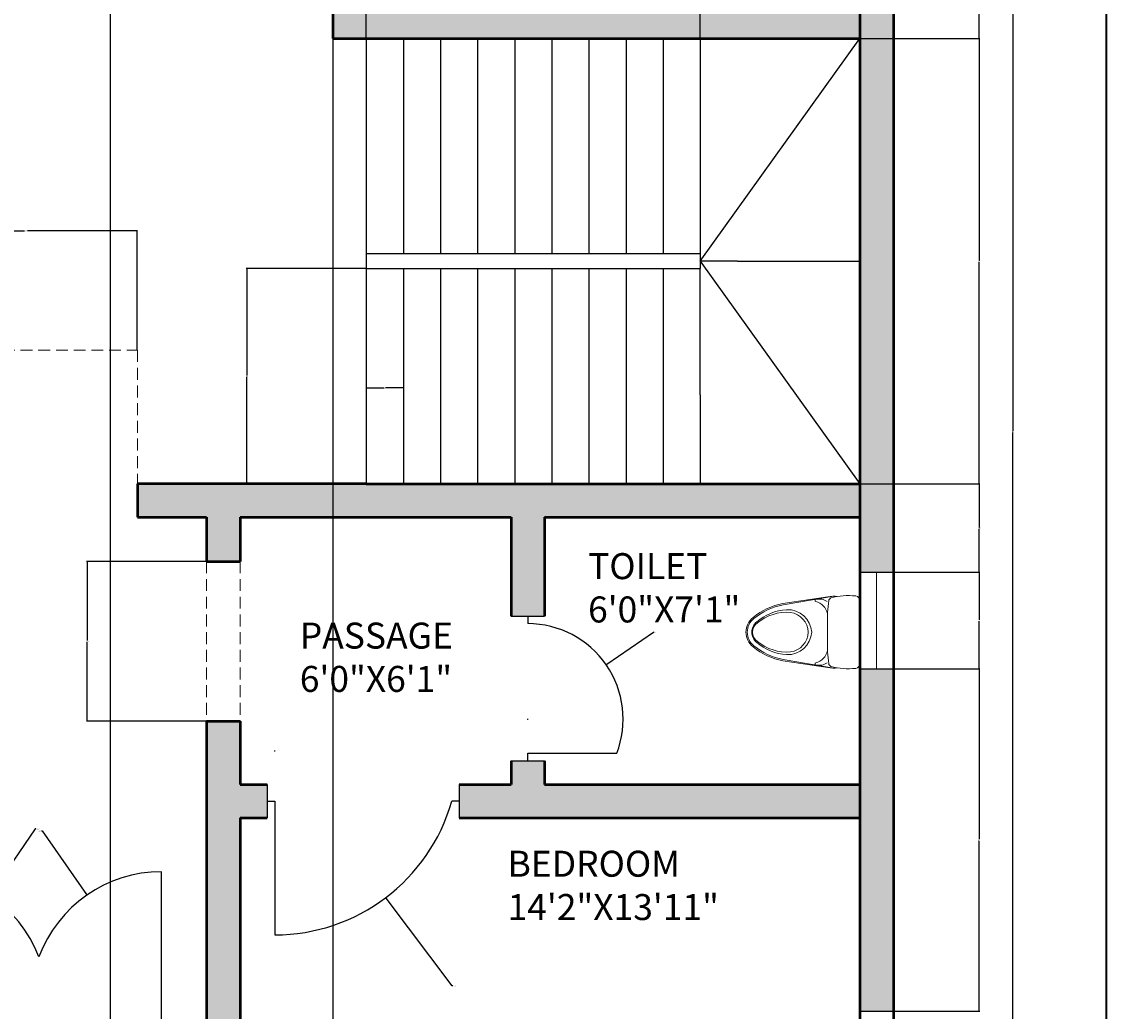
# Model space of a CAD drawing. Units: inches. Extents: x 1676 to 2199, y 1657 to 2783.
# Tile 7 of 10: x 1907 to 2199, y 1905 to 2172. Entities that reach past the tile are written whole.
import ezdxf

# ---------------------------------------------------------------- set-up
doc = ezdxf.new("R2010")
doc.units = ezdxf.units.IN
doc.linetypes.add('HIDDEN2', pattern=[4.7625, 3.175, -1.5875])
for name, color, linetype, lineweight in [('A-ANNO-DIMS', 2, 'Continuous', 18), ('A-ANNO-TTLB', 7, 'Continuous', 35), ('A-AREA-IDEN', 7, 'Continuous', 18), ('A-DOOR', 4, 'Continuous', 25), ('A-FLOR-FIXT', 9, 'Continuous', 18), ('A-FLOR-STRS', 7, 'Continuous', 25), ('A-GLAZ', 4, 'Continuous', 18), ('A-WALL', 7, 'Continuous', 50), ('A-WALL-HIDN', 253, 'HIDDEN2', 18)]:
    doc.layers.add(name, color=color, linetype=linetype, lineweight=lineweight)
doc.layers.add('A-WALL-PATT', color=251, linetype='Continuous', lineweight=13, true_color=0x636466)
doc.styles.get("Standard").update_dxf_attribs({"font": 'arial.ttf'})
doc.dimstyles.get("Standard").update_dxf_attribs({"dimtxt": 0.18, "dimasz": 0.18, "dimexe": 0.18, "dimexo": 0.0625, "dimgap": 0.09, "dimtad": 0, "dimtih": 1, "dimtoh": 1, "dimdec": 4, "dimzin": 0, "dimdsep": 46, "dimtxsty": 'Standard', "dimcen": 0.09, "dimadec": 0, "dimazin": 0, "dimtfac": 1, "dimtdec": 4, "dimtofl": 0, "dimtmove": 0, "dimatfit": 3, "dimfxl": 1, "dimtolj": 1, "dimtzin": 0, "dimarcsym": 0})

# ---------------------------------------------------------------- blocks, each defined once
blk = doc.blocks.new('A$C188A4A68')
at = {"ltscale": 20}
for p, q in [((0.2444, 0.7693), (0.0344, 0.7693)), ((0.2444, 0.7693), (0.4544, 0.7693)), ((0.0013, 0.5938), (0.0607, 0.2504)), ((0.4874, 0.5938), (0.428, 0.2504)), ((0.0054, 0.5515), (0.0519, 0.2489)), ((0.2444, 0.5498), (0.1889, 0.5498)), ((0.2444, 0.5498), (0.2998, 0.5498)), ((0.4833, 0.5515), (0.4368, 0.2489))]:
    blk.add_line(p, q, dxfattribs=at)
for centre, radius, start, end in [((0.442, 0.6914), 0.4447, 173.63949, 195.46404), ((0.0344, 0.7343), 0.0349, 90, 169.59261), ((0.4544, 0.7343), 0.0349, 10.40739, 90), ((0.0467, 0.6914), 0.4447, 344.53596, 6.36051), ((0.2125, 0.5932), 0.2113, 172.64979, 191.36585), ((0.2762, 0.5932), 0.2113, 348.63415, 7.35021), ((0.0333, 0.5802), 0.0213, 200.24298, 267.15028), ((0.1303, 0.4913), 0.1097, 148.50689, 190.04883), ((0.1632, 1.4554), 0.906, 261.69023, 271.62576), ((0.1461, 0.4405), 0.1134, 104.10408, 164.15012), ((0.3255, 1.4554), 0.906, 268.37424, 278.30977), ((0.3426, 0.4405), 0.1134, 15.84988, 75.89592), ((0.3584, 0.4913), 0.1097, 349.95117, 31.49311), ((0.4554, 0.5802), 0.0213, 272.84972, 339.75702), ((0.0297, 0.4734), 0.0075, 189.82636, 345.08753), ((0.254, 0.2824), 0.1613, 93.43328, 183.00378), ((0.2347, 0.2824), 0.1613, 356.99622, 86.56672), ((0.459, 0.4734), 0.0075, 194.91247, 350.17364), ((0.2493, 0.2813), 0.1393, 92.03292, 172.03731), ((0.2394, 0.2813), 0.1393, 7.96269, 87.96708), ((0.4211, 0.2752), 0.3108, 175.32131, 219.24773), ((0.0676, 0.2752), 0.3108, 320.75227, 4.67869), ((0.4781, 0.3243), 0.4328, 190.02971, 219.74275), ((0.4781, 0.3243), 0.4238, 190.04347, 219.7538), ((0.4311, 0.2946), 0.3389, 183.50421, 221.02292), ((0.0576, 0.2946), 0.3389, 318.97708, 356.49579), ((0.0106, 0.3243), 0.4238, 320.2462, 349.95653), ((0.0106, 0.3243), 0.4328, 320.25725, 349.97029), ((0.2498, 0.1282), 0.0854, 215.56846, 266.31968), ((0.2389, 0.1282), 0.0854, 273.68032, 324.43154), ((0.2444, 0.127), 0.127, 218.71605, 270), ((0.2444, 0.127), 0.118, 218.67741, 270), ((0.2444, 0.127), 0.088, 218.504, 270), ((0.2444, 0.127), 0.088, 270, 321.496), ((0.2444, 0.127), 0.118, 270, 321.32259), ((0.2444, 0.127), 0.127, 270, 321.28395)]:
    blk.add_arc(centre, radius, start, end, dxfattribs=at)
blk = doc.blocks.new('*D20')
at = {"layer": 'A-ANNO-DIMS', "color": 0, "lineweight": -2, "transparency": 16777216}
for p, q in [((2142.14, 2341.09), (2174.4, 2341.09)), ((2174.22, 2340.91), (2174.22, 2061.27)), ((2174.22, 1781.27), (2174.22, 2060.91)), ((2142.14, 1781.09), (2174.4, 1781.09))]:
    blk.add_line(p, q, dxfattribs=at)
at = {"layer": 'A-ANNO-DIMS', "color": 0, "transparency": 16777216}
for points in [[(2174.19, 2340.91), (2174.25, 2340.91), (2174.22, 2341.09)], [(2174.19, 1781.27), (2174.25, 1781.27), (2174.22, 1781.09)]]:
    blk.add_solid(points, dxfattribs=at)
at = {"layer": 'Defpoints', "color": 0, "transparency": 16777216}
for p in [(2142.07, 2341.09), (2174.22, 2341.09), (2142.07, 1781.09)]:
    blk.add_point(p, dxfattribs=at)
at = {"layer": 'A-ANNO-DIMS', "color": 0, "transparency": 16777216, "insert": (2174.22, 2061.09), "char_height": 0.18, "attachment_point": 5}
blk.add_mtext('\\A1;560', dxfattribs=at)
blk = doc.blocks.new('*D31')
at = {"layer": 'A-ANNO-DIMS', "color": 0, "lineweight": -2, "transparency": 16777216}
for p, q in [((2133.14, 1997.28), (2165.4, 1997.28)), ((2165.22, 1997.1), (2165.22, 1951.32)), ((2165.22, 1905.17), (2165.22, 1950.95)), ((2133.14, 1904.99), (2165.4, 1904.99))]:
    blk.add_line(p, q, dxfattribs=at)
at = {"layer": 'A-ANNO-DIMS', "color": 0, "transparency": 16777216}
for points in [[(2165.19, 1997.1), (2165.25, 1997.1), (2165.22, 1997.28)], [(2165.19, 1905.17), (2165.25, 1905.17), (2165.22, 1904.99)]]:
    blk.add_solid(points, dxfattribs=at)
at = {"layer": 'Defpoints', "color": 0, "transparency": 16777216}
for p in [(2133.07, 1997.28), (2133.07, 1904.99), (2165.22, 1904.99)]:
    blk.add_point(p, dxfattribs=at)
at = {"layer": 'A-ANNO-DIMS', "color": 0, "transparency": 16777216, "insert": (2165.22, 1951.13), "char_height": 0.18, "attachment_point": 5}
blk.add_mtext('\\A1;92.29', dxfattribs=at)
blk = doc.blocks.new('*D32')
at = {"layer": 'A-ANNO-DIMS', "color": 0, "lineweight": -2, "transparency": 16777216}
for p, q in [((2133.14, 2023.28), (2165.4, 2023.28)), ((2165.22, 2023.1), (2165.22, 2010.46)), ((2165.22, 1997.46), (2165.22, 2010.1)), ((2133.14, 1997.28), (2165.4, 1997.28))]:
    blk.add_line(p, q, dxfattribs=at)
at = {"layer": 'A-ANNO-DIMS', "color": 0, "transparency": 16777216}
for points in [[(2165.19, 2023.1), (2165.25, 2023.1), (2165.22, 2023.28)], [(2165.19, 1997.46), (2165.25, 1997.46), (2165.22, 1997.28)]]:
    blk.add_solid(points, dxfattribs=at)
at = {"layer": 'Defpoints', "color": 0, "transparency": 16777216}
for p in [(2133.07, 2023.28), (2133.07, 1997.28), (2165.22, 1997.28)]:
    blk.add_point(p, dxfattribs=at)
at = {"layer": 'A-ANNO-DIMS', "color": 0, "transparency": 16777216, "insert": (2165.22, 2010.28), "char_height": 0.18, "attachment_point": 5}
blk.add_mtext('\\A1;26', dxfattribs=at)
blk = doc.blocks.new('*D33')
at = {"layer": 'A-ANNO-DIMS', "color": 0, "lineweight": -2, "transparency": 16777216}
for p, q in [((2133.14, 2047.09), (2165.4, 2047.09)), ((2165.22, 2046.91), (2165.22, 2035.36)), ((2165.22, 2023.46), (2165.22, 2035)), ((2133.14, 2023.28), (2165.4, 2023.28))]:
    blk.add_line(p, q, dxfattribs=at)
at = {"layer": 'A-ANNO-DIMS', "color": 0, "transparency": 16777216}
for points in [[(2165.19, 2046.91), (2165.25, 2046.91), (2165.22, 2047.09)], [(2165.19, 2023.46), (2165.25, 2023.46), (2165.22, 2023.28)]]:
    blk.add_solid(points, dxfattribs=at)
at = {"layer": 'Defpoints', "color": 0, "transparency": 16777216}
for p in [(2133.07, 2047.09), (2133.07, 2023.28), (2165.22, 2023.28)]:
    blk.add_point(p, dxfattribs=at)
at = {"layer": 'A-ANNO-DIMS', "color": 0, "transparency": 16777216, "insert": (2165.22, 2035.18), "char_height": 0.18, "attachment_point": 5}
blk.add_mtext('\\A1;23.81', dxfattribs=at)
blk = doc.blocks.new('*D34')
at = {"layer": 'A-ANNO-DIMS', "color": 0, "lineweight": -2, "transparency": 16777216}
for p, q in [((2133.14, 2167.09), (2165.4, 2167.09)), ((2165.22, 2166.91), (2165.22, 2107.27)), ((2165.22, 2047.27), (2165.22, 2106.91)), ((2133.14, 2047.09), (2165.4, 2047.09))]:
    blk.add_line(p, q, dxfattribs=at)
at = {"layer": 'A-ANNO-DIMS', "color": 0, "transparency": 16777216}
for points in [[(2165.19, 2166.91), (2165.25, 2166.91), (2165.22, 2167.09)], [(2165.19, 2047.27), (2165.25, 2047.27), (2165.22, 2047.09)]]:
    blk.add_solid(points, dxfattribs=at)
at = {"layer": 'Defpoints', "color": 0, "transparency": 16777216}
for p in [(2133.07, 2167.09), (2133.07, 2047.09), (2165.22, 2047.09)]:
    blk.add_point(p, dxfattribs=at)
at = {"layer": 'A-ANNO-DIMS', "color": 0, "transparency": 16777216, "insert": (2165.22, 2107.09), "char_height": 0.18, "attachment_point": 5}
blk.add_mtext('\\A1;120', dxfattribs=at)
blk = doc.blocks.new('*D35')
at = {"layer": 'A-ANNO-DIMS', "color": 0, "lineweight": -2, "transparency": 16777216}
for p, q in [((2133.14, 2238.21), (2165.4, 2238.21)), ((2165.22, 2238.03), (2165.22, 2202.83)), ((2165.22, 2167.27), (2165.22, 2202.47)), ((2133.14, 2167.09), (2165.4, 2167.09))]:
    blk.add_line(p, q, dxfattribs=at)
at = {"layer": 'A-ANNO-DIMS', "color": 0, "transparency": 16777216}
for points in [[(2165.19, 2238.03), (2165.25, 2238.03), (2165.22, 2238.21)], [(2165.19, 2167.27), (2165.25, 2167.27), (2165.22, 2167.09)]]:
    blk.add_solid(points, dxfattribs=at)
at = {"layer": 'Defpoints', "color": 0, "transparency": 16777216}
for p in [(2133.07, 2238.21), (2133.07, 2167.09), (2165.22, 2167.09)]:
    blk.add_point(p, dxfattribs=at)
at = {"layer": 'A-ANNO-DIMS', "color": 0, "transparency": 16777216, "insert": (2165.22, 2202.65), "char_height": 0.18, "attachment_point": 5}
blk.add_mtext('\\A1;71.12', dxfattribs=at)
blk = doc.blocks.new('*D40')
at = {"layer": 'A-ANNO-DIMS', "color": 0, "lineweight": -2, "transparency": 16777216}
for p, q in [((1931.07, 2236.02), (1931.07, 1695.28)), ((1991.07, 2236.02), (1991.07, 1695.28)), ((1931.25, 1695.46), (1960.86, 1695.46)), ((1990.89, 1695.46), (1961.29, 1695.46))]:
    blk.add_line(p, q, dxfattribs=at)
at = {"layer": 'A-ANNO-DIMS', "color": 0, "transparency": 16777216}
for points in [[(1931.25, 1695.49), (1931.25, 1695.43), (1931.07, 1695.46)], [(1990.89, 1695.49), (1990.89, 1695.43), (1991.07, 1695.46)]]:
    blk.add_solid(points, dxfattribs=at)
at = {"layer": 'Defpoints', "color": 0, "transparency": 16777216}
for p in [(1931.07, 2236.09), (1991.07, 2236.09), (1991.07, 1695.46)]:
    blk.add_point(p, dxfattribs=at)
at = {"layer": 'A-ANNO-DIMS', "color": 0, "transparency": 16777216, "insert": (1961.07, 1695.46), "char_height": 0.18, "attachment_point": 5}
blk.add_mtext('\\A1;60', dxfattribs=at)
blk = doc.blocks.new('*D45')
at = {"layer": 'A-ANNO-DIMS', "color": 0, "lineweight": -2, "transparency": 16777216}
for p, q in [((2000.07, 2167.15), (2000.07, 2199.42)), ((2000.25, 2199.24), (2044.86, 2199.24)), ((2089.89, 2199.24), (2045.29, 2199.24)), ((2090.07, 2167.15), (2090.07, 2199.42))]:
    blk.add_line(p, q, dxfattribs=at)
at = {"layer": 'A-ANNO-DIMS', "color": 0, "transparency": 16777216}
for points in [[(2000.25, 2199.27), (2000.25, 2199.21), (2000.07, 2199.24)], [(2089.89, 2199.27), (2089.89, 2199.21), (2090.07, 2199.24)]]:
    blk.add_solid(points, dxfattribs=at)
at = {"layer": 'Defpoints', "color": 0, "transparency": 16777216}
for p in [(2090.07, 2199.24), (2000.07, 2167.09), (2090.07, 2167.09)]:
    blk.add_point(p, dxfattribs=at)
at = {"layer": 'A-ANNO-DIMS', "color": 0, "transparency": 16777216, "insert": (2045.07, 2199.24), "char_height": 0.18, "attachment_point": 5}
blk.add_mtext('\\A1;90', dxfattribs=at)
blk = doc.blocks.new('*D46')
at = {"layer": 'A-ANNO-DIMS', "color": 0, "lineweight": -2, "transparency": 16777216}
for p, q in [((2090.07, 2167.15), (2090.07, 2199.42)), ((2090.25, 2199.24), (2111.35, 2199.24)), ((2132.89, 2199.24), (2111.8, 2199.24)), ((2133.07, 2167.15), (2133.07, 2199.42))]:
    blk.add_line(p, q, dxfattribs=at)
at = {"layer": 'A-ANNO-DIMS', "color": 0, "transparency": 16777216}
for points in [[(2090.25, 2199.27), (2090.25, 2199.21), (2090.07, 2199.24)], [(2132.89, 2199.27), (2132.89, 2199.21), (2133.07, 2199.24)]]:
    blk.add_solid(points, dxfattribs=at)
at = {"layer": 'Defpoints', "color": 0, "transparency": 16777216}
for p in [(2133.07, 2199.24), (2090.07, 2167.09), (2133.07, 2167.09)]:
    blk.add_point(p, dxfattribs=at)
at = {"layer": 'A-ANNO-DIMS', "color": 0, "transparency": 16777216, "insert": (2111.57, 2199.24), "char_height": 0.18, "attachment_point": 5}
blk.add_mtext('\\A1;43', dxfattribs=at)
blk = doc.blocks.new('*D47')
at = {"layer": 'A-ANNO-DIMS', "color": 0, "lineweight": -2, "transparency": 16777216}
for p, q in [((2000.01, 2105.09), (1967.74, 2105.09)), ((1967.92, 2104.91), (1967.92, 2076.27)), ((1967.92, 2047.27), (1967.92, 2075.91)), ((2000.01, 2047.09), (1967.74, 2047.09))]:
    blk.add_line(p, q, dxfattribs=at)
at = {"layer": 'A-ANNO-DIMS', "color": 0, "transparency": 16777216}
for points in [[(1967.89, 2104.91), (1967.95, 2104.91), (1967.92, 2105.09)], [(1967.89, 2047.27), (1967.95, 2047.27), (1967.92, 2047.09)]]:
    blk.add_solid(points, dxfattribs=at)
at = {"layer": 'Defpoints', "color": 0, "transparency": 16777216}
for p in [(1967.92, 2105.09), (2000.07, 2105.09), (2000.07, 2047.09)]:
    blk.add_point(p, dxfattribs=at)
at = {"layer": 'A-ANNO-DIMS', "color": 0, "transparency": 16777216, "insert": (1967.92, 2076.09), "char_height": 0.18, "attachment_point": 5}
blk.add_mtext('\\A1;58', dxfattribs=at)
blk = doc.blocks.new('*D48')
at = {"layer": 'A-ANNO-DIMS', "color": 0, "lineweight": -2, "transparency": 16777216}
for p, q in [((2000.07, 2105.02), (2000.07, 2072.76)), ((2010.07, 2105.02), (2010.07, 2072.76)), ((2000.25, 2072.94), (2004.86, 2072.94)), ((2009.89, 2072.94), (2005.29, 2072.94))]:
    blk.add_line(p, q, dxfattribs=at)
at = {"layer": 'A-ANNO-DIMS', "color": 0, "transparency": 16777216}
for points in [[(2000.25, 2072.97), (2000.25, 2072.91), (2000.07, 2072.94)], [(2009.89, 2072.97), (2009.89, 2072.91), (2010.07, 2072.94)]]:
    blk.add_solid(points, dxfattribs=at)
at = {"layer": 'Defpoints', "color": 0, "transparency": 16777216}
for p in [(2000.07, 2105.09), (2010.07, 2105.09), (2000.07, 2072.94)]:
    blk.add_point(p, dxfattribs=at)
at = {"layer": 'A-ANNO-DIMS', "color": 0, "transparency": 16777216, "insert": (2005.07, 2072.94), "char_height": 0.18, "attachment_point": 5}
blk.add_mtext('\\A1;10', dxfattribs=at)
blk = doc.blocks.new('*D49')
at = {"layer": 'A-ANNO-DIMS', "color": 0, "lineweight": -2, "transparency": 16777216}
for p, q in [((1878.39, 2083.15), (1878.39, 2115.42)), ((1878.57, 2115.24), (1908.02, 2115.24)), ((1938.22, 2115.24), (1908.78, 2115.24)), ((1938.4, 2083.15), (1938.4, 2115.42))]:
    blk.add_line(p, q, dxfattribs=at)
at = {"layer": 'A-ANNO-DIMS', "color": 0, "transparency": 16777216}
for points in [[(1878.57, 2115.27), (1878.57, 2115.21), (1878.39, 2115.24)], [(1938.22, 2115.27), (1938.22, 2115.21), (1938.4, 2115.24)]]:
    blk.add_solid(points, dxfattribs=at)
at = {"layer": 'Defpoints', "color": 0, "transparency": 16777216}
for p in [(1938.4, 2115.24), (1878.39, 2083.09), (1938.4, 2083.09)]:
    blk.add_point(p, dxfattribs=at)
at = {"layer": 'A-ANNO-DIMS', "color": 0, "transparency": 16777216, "insert": (1908.4, 2115.24), "char_height": 0.18, "attachment_point": 5}
blk.add_mtext('\\A1;60.01', dxfattribs=at)
blk = doc.blocks.new('*D58')
at = {"layer": 'A-ANNO-DIMS', "color": 0, "lineweight": -2, "transparency": 16777216}
for p, q in [((1957.01, 2026.16), (1924.74, 2026.16)), ((1924.92, 2025.98), (1924.92, 2004.84)), ((1924.92, 1983.33), (1924.92, 2004.47)), ((1957.01, 1983.15), (1924.74, 1983.15))]:
    blk.add_line(p, q, dxfattribs=at)
at = {"layer": 'A-ANNO-DIMS', "color": 0, "transparency": 16777216}
for points in [[(1924.89, 2025.98), (1924.95, 2025.98), (1924.92, 2026.16)], [(1924.89, 1983.33), (1924.95, 1983.33), (1924.92, 1983.15)]]:
    blk.add_solid(points, dxfattribs=at)
at = {"layer": 'Defpoints', "color": 0, "transparency": 16777216}
for p in [(1924.92, 2026.16), (1957.07, 2026.16), (1957.07, 1983.15)]:
    blk.add_point(p, dxfattribs=at)
at = {"layer": 'A-ANNO-DIMS', "color": 0, "transparency": 16777216, "insert": (1924.92, 2004.66), "char_height": 0.18, "attachment_point": 5}
blk.add_mtext('\\A1;43.01', dxfattribs=at)
blk = doc.blocks.new('*D79')
at = {"layer": 'A-ANNO-DIMS', "color": 0, "lineweight": -2, "transparency": 16777216}
for p, q in [((2077.47, 2007.01), (2064.91, 1998.38)), ((2077.65, 2007.01), (2077.47, 2007.01)), ((2043.48, 1983.71), (2043.66, 1983.71)), ((2043.57, 1983.62), (2043.57, 1983.8))]:
    blk.add_line(p, q, dxfattribs=at)
at = {"layer": 'A-ANNO-DIMS', "color": 0, "transparency": 16777216}
blk.add_solid([(2064.89, 1998.4), (2064.93, 1998.35), (2064.76, 1998.28)], dxfattribs=at)
at = {"layer": 'Defpoints', "color": 0, "transparency": 16777216}
for p in [(2064.76, 1998.28), (2043.57, 1983.71)]:
    blk.add_point(p, dxfattribs=at)
at = {"layer": 'A-ANNO-DIMS', "color": 0, "transparency": 16777216, "insert": (2078.2, 2007.01), "char_height": 0.18, "attachment_point": 5}
blk.add_mtext('\\A1;R25.707', dxfattribs=at)
blk = doc.blocks.new('*D80')
at = {"layer": 'A-ANNO-DIMS', "color": 0, "lineweight": -2, "transparency": 16777216}
for p, q in [((1975.33, 1975.17), (1975.51, 1975.17)), ((1975.42, 1975.08), (1975.42, 1975.26)), ((2023.22, 1911.85), (2005.4, 1935.45)), ((2023.4, 1911.85), (2023.22, 1911.85))]:
    blk.add_line(p, q, dxfattribs=at)
at = {"layer": 'A-ANNO-DIMS', "color": 0, "transparency": 16777216}
blk.add_solid([(2005.43, 1935.47), (2005.38, 1935.44), (2005.29, 1935.6)], dxfattribs=at)
at = {"layer": 'Defpoints', "color": 0, "transparency": 16777216}
for p in [(1975.42, 1975.17), (2005.29, 1935.6)]:
    blk.add_point(p, dxfattribs=at)
at = {"layer": 'A-ANNO-DIMS', "color": 0, "transparency": 16777216, "insert": (2023.88, 1911.85), "char_height": 0.18, "attachment_point": 5}
blk.add_mtext('\\A1;R49.59', dxfattribs=at)
blk = doc.blocks.new('*D81')
at = {"layer": 'A-ANNO-DIMS', "color": 0, "lineweight": -2, "transparency": 16777216}
for p, q in [((1910.86, 1954.14), (1898.76, 1936.45)), ((1911.04, 1954.14), (1910.86, 1954.14)), ((1878.23, 1906.55), (1878.41, 1906.55)), ((1878.32, 1906.46), (1878.32, 1906.64))]:
    blk.add_line(p, q, dxfattribs=at)
at = {"layer": 'A-ANNO-DIMS', "color": 0, "transparency": 16777216}
blk.add_solid([(1898.73, 1936.46), (1898.78, 1936.43), (1898.66, 1936.3)], dxfattribs=at)
at = {"layer": 'Defpoints', "color": 0, "transparency": 16777216}
for p in [(1898.66, 1936.3), (1878.32, 1906.55)]:
    blk.add_point(p, dxfattribs=at)
at = {"layer": 'A-ANNO-DIMS', "color": 0, "transparency": 16777216, "insert": (1911.59, 1954.14), "char_height": 0.18, "attachment_point": 5}
blk.add_mtext('\\A1;R36.034', dxfattribs=at)
blk = doc.blocks.new('*D82')
at = {"layer": 'A-ANNO-DIMS', "color": 0, "lineweight": -2, "transparency": 16777216}
for p, q in [((1912.55, 1953.6), (1912.73, 1953.6)), ((1912.73, 1953.6), (1924.68, 1936.43)), ((1944.79, 1907.42), (1944.97, 1907.42)), ((1944.88, 1907.33), (1944.88, 1907.51))]:
    blk.add_line(p, q, dxfattribs=at)
at = {"layer": 'A-ANNO-DIMS', "color": 0, "transparency": 16777216}
blk.add_solid([(1924.71, 1936.45), (1924.66, 1936.41), (1924.78, 1936.28)], dxfattribs=at)
at = {"layer": 'Defpoints', "color": 0, "transparency": 16777216}
for p in [(1924.78, 1936.28), (1944.88, 1907.42)]:
    blk.add_point(p, dxfattribs=at)
at = {"layer": 'A-ANNO-DIMS', "color": 0, "transparency": 16777216, "insert": (1912.07, 1953.6), "char_height": 0.18, "attachment_point": 5}
blk.add_mtext('\\A1;R35.17', dxfattribs=at)

msp = doc.modelspace()

# ---------------------------------------------------------------- hatches: boundary and pattern name
at = {"layer": 'A-WALL-PATT'}
h = msp.add_hatch(color=256, dxfattribs=at)
h.dxf.hatch_style = 1
h.paths.add_polyline_path([(1945.4216, 2336.5871), (1945.4216, 2341.0871), (1755.075, 2341.0871), (1755.075, 2323.0739), (1764.075, 2323.0739), (1764.075, 2332.0871), (1945.4216, 2332.0871)])
h.paths.add_polyline_path([(1764.075, 2299.0739), (1755.075, 2299.0739), (1755.075, 2266.2601), (1759.575, 2266.2601), (1764.075, 2266.2601)])
h.paths.add_polyline_path([(1843.075, 2285.0871), (1764.075, 2285.0871), (1764.075, 2276.0871), (1843.075, 2276.0871)])
h.paths.add_polyline_path([(1931.075, 2332.0871), (1922.075, 2332.0871), (1922.075, 2285.0871), (1907.247, 2285.0871), (1907.247, 2276.0871), (1922.075, 2276.0871), (1922.075, 2263.0871), (1922.075, 2214.434), (1922.075, 2183.2198), (1931.075, 2183.2198), (1931.075, 2214.434), (1931.075, 2227.0871), (1991.075, 2227.0871), (1991.075, 2176.0871), (1991.075, 2167.0871), (2000.075, 2167.0871), (2133.075, 2167.0871), (2133.075, 2176.0871), (2000.075, 2176.0871), (2000.075, 2245.3418), (1995.575, 2245.3418), (1991.075, 2245.3418), (1991.075, 2236.0871), (1931.075, 2236.0871)])
h.paths.add_polyline_path([(2000.075, 2332.0871), (1991.075, 2332.0871), (1991.075, 2285.0871), (1991.075, 2274.6339), (2000.075, 2274.6339), (2000.075, 2285.0871)], flags=17)
h.paths.add_polyline_path([(2142.075, 2341.0871), (1969.4216, 2341.0871), (1969.4216, 2332.0871), (2133.075, 2332.0871), (2133.075, 2298.2101), (2142.075, 2298.2101)])
h.paths.add_polyline_path([(2142.075, 1844.9908), (2133.075, 1844.9908), (2133.075, 1790.0871), (2061.2106, 1790.0871), (2061.2106, 1781.0871), (2142.075, 1781.0871)])
h.paths.add_polyline_path([(2001.2106, 1790.0871), (1966.075, 1790.0871), (1966.075, 1957.0871), (1973.4183, 1957.0871), (1973.4183, 1966.0871), (1966.075, 1966.0871), (1966.075, 1983.1515), (1957.075, 1983.1515), (1957.075, 1899.0871), (1946.8789, 1899.0871), (1946.8789, 1890.0871), (1957.075, 1890.0871), (1957.075, 1781.0871), (2001.2106, 1781.0871), (2001.2106, 1785.5871)])
h.paths.add_polyline_path([(1876.3163, 1894.5871), (1876.3163, 1899.0871), (1820.9237, 1899.0871), (1820.9237, 1890.0871), (1876.3163, 1890.0871)])
h.paths.add_polyline_path([(1764.075, 2093.9207), (1759.575, 2093.9207), (1755.075, 2093.9207), (1755.075, 2019.5723), (1764.075, 2019.5723)])
h.paths.add_polyline_path([(1878.3926, 2083.0871), (1764.075, 2083.0871), (1764.075, 2074.0871), (1878.3926, 2074.0871)])
h.paths.add_polyline_path([(1764.075, 1959.5723), (1755.075, 1959.5723), (1755.075, 1890.0871), (1784.9237, 1890.0871), (1784.9237, 1894.5871), (1784.9237, 1899.0871), (1764.075, 1899.0871)])
h.paths.add_polyline_path([(2133.075, 2047.0871), (2000.075, 2047.0871), (1966.075, 2047.0871), (1957.075, 2047.0871), (1938.4046, 2047.0871), (1938.4046, 2038.0871), (1957.075, 2038.0871), (1957.075, 2026.1604), (1966.075, 2026.1604), (1966.075, 2038.0871), (2039.075, 2038.0871), (2039.075, 2011.4216), (2048.075, 2011.4216), (2048.075, 2038.0871), (2133.075, 2038.0871)])
h.paths.add_polyline_path([(2133.075, 1966.0871), (2048.075, 1966.0871), (2048.075, 1972.5045), (2039.075, 1972.5045), (2039.075, 1966.0871), (2025.1075, 1966.0871), (2025.1075, 1957.0871), (2133.075, 1957.0871)])
h.paths.add_polyline_path([(1764.075, 2206.2601), (1755.075, 2206.2601), (1755.075, 2153.9207), (1764.075, 2153.9207)])
h = msp.add_hatch(color=256, dxfattribs=at)
h.dxf.hatch_style = 1
h.paths.add_polyline_path([(2142.075, 2238.2101), (2133.075, 2238.2101), (2133.075, 2023.2789), (2142.075, 2023.2789)])
h.paths.add_polyline_path([(2142.075, 1997.2789), (2133.075, 1997.2789), (2133.075, 1904.9908), (2142.075, 1904.9908)])

# ---------------------------------------------------------------- linework, layer by layer
at = {"layer": 'A-ANNO-TTLB'}
msp.add_lwpolyline([(1676.2722, 2782.5054), (2199.4461, 2782.5054), (2199.4461, 1657.2705), (1676.2722, 1657.2705)], close=True, dxfattribs=at)
at = {"layer": 'A-DOOR'}
for p, q in [((2039.075, 2011.4216), (2048.075, 2011.4216)), ((2043.575, 2011.4216), (2043.575, 2009.4216)), ((2039.075, 1972.5045), (2048.075, 1972.5045)), ((2043.575, 1972.5045), (2043.575, 1974.5045)), ((2043.575, 1974.5045), (2067.575, 1974.5045)), ((1973.4183, 1966.0871), (1973.4183, 1957.0871)), ((2025.1075, 1966.0871), (2025.1075, 1957.0871)), ((1973.4183, 1961.5871), (1975.4183, 1961.5871)), ((1975.4183, 1961.5871), (1975.4183, 1925.5871)), ((2025.1075, 1961.5871), (2023.1075, 1961.5871)), ((1944.8789, 1894.5871), (1944.8789, 1942.5871))]:
    msp.add_line(p, q, dxfattribs=at)
for centre, radius, start, end in [((2043.575, 1983.7149), 25.7066, 339.004859, 90), ((1975.4183, 1975.174), 49.5869, 270, 344.097464), ((1878.3163, 1906.5528), 36.0343, 21.266188, 90), ((1944.8789, 1907.4201), 35.1669, 90, 159.697131)]:
    msp.add_arc(centre, radius, start, end, dxfattribs=at)
at = {"layer": 'A-FLOR-STRS'}
for p, q in [((2000.075, 2167.0871), (2000.075, 2071.0871)), ((2000.075, 2167.0871), (2000.075, 2107.0871)), ((2010.075, 2167.0871), (2010.075, 2109.0871)), ((2010.075, 2167.0871), (2010.075, 2109.0871)), ((2020.075, 2167.0871), (2020.075, 2109.0871)), ((2030.075, 2167.0871), (2030.075, 2109.0871)), ((2040.075, 2167.0871), (2040.075, 2109.0871)), ((2050.075, 2167.0871), (2050.075, 2109.0871)), ((2060.075, 2167.0871), (2060.075, 2109.0871)), ((2070.075, 2167.0871), (2070.075, 2109.0871)), ((2080.075, 2167.0871), (2080.075, 2109.0871)), ((2090.075, 2167.0871), (2090.075, 2109.0871)), ((2090.075, 2107.0871), (2133.075, 2167.0871)), ((2090.075, 2109.0871), (2000.075, 2109.0871)), ((2000.075, 2107.0871), (2000.075, 2105.0871)), ((2090.075, 2109.0871), (2090.075, 2105.0871)), ((2100.075, 2107.0871), (2090.075, 2107.0871)), ((2090.075, 2107.0871), (2133.075, 2047.0871)), ((2100.075, 2107.0871), (2133.075, 2107.0871)), ((2000.075, 2105.0871), (2090.075, 2105.0871)), ((2010.075, 2105.0871), (2010.075, 2071.0871)), ((2020.075, 2105.0871), (2020.075, 2047.0871)), ((2030.075, 2105.0871), (2030.075, 2047.0871)), ((2040.075, 2105.0871), (2040.075, 2047.0871)), ((2050.075, 2105.0871), (2050.075, 2047.0871)), ((2060.075, 2105.0871), (2060.075, 2047.0871)), ((2070.075, 2105.0871), (2070.075, 2047.0871)), ((2080.075, 2105.0871), (2080.075, 2047.0871)), ((2090.075, 2071.0871), (2090.075, 2105.0871)), ((2000.075, 2071.0871), (2000.075, 2047.0871)), ((2010.075, 2071.0871), (2010.075, 2047.0871)), ((2090.075, 2071.0871), (2090.075, 2047.0871))]:
    msp.add_line(p, q, dxfattribs=at)
at = {"layer": 'A-GLAZ'}
for p, q in [((2133.075, 2023.2789), (2142.075, 2023.2789)), ((2142.075, 2023.2789), (2137.575, 2023.2789)), ((2137.575, 2023.2789), (2137.575, 2021.2789)), ((2137.575, 2021.2789), (2137.575, 1997.2789)), ((2137.575, 1997.2789), (2133.075, 1997.2789)), ((2133.075, 1997.2789), (2142.075, 1997.2789))]:
    msp.add_line(p, q, dxfattribs=at)
at = {"layer": 'A-WALL'}
for p, q in [((2142.075, 2341.0871), (2142.075, 1781.0871)), ((2133.075, 2332.0871), (2133.075, 1790.0871)), ((1991.075, 2176.0871), (1991.075, 2167.0871)), ((1991.075, 2167.0871), (2000.075, 2167.0871)), ((2000.075, 2167.0871), (2133.075, 2167.0871)), ((1957.075, 2047.0871), (1938.4046, 2047.0871)), ((1938.4046, 2047.0871), (1938.4046, 2038.0871)), ((1966.075, 2047.0871), (1957.075, 2047.0871)), ((2000.075, 2047.0871), (1966.075, 2047.0871)), ((2000.075, 2047.0871), (2133.075, 2047.0871)), ((1938.4046, 2038.0871), (1957.075, 2038.0871)), ((1957.075, 2038.0871), (1957.075, 2026.1604)), ((1966.075, 2038.0871), (2039.075, 2038.0871)), ((1966.075, 2038.0871), (1966.075, 2026.1604)), ((1966.075, 2038.0871), (1966.075, 2026.1604)), ((1966.075, 2038.0871), (1966.075, 2038.0871)), ((1966.075, 2038.0871), (1966.075, 2026.1604)), ((2039.075, 2038.0871), (2039.075, 2011.4216)), ((2048.075, 2038.0871), (2048.075, 2011.4216)), ((2048.075, 2038.0871), (2133.075, 2038.0871)), ((1957.075, 2026.1604), (1966.075, 2026.1604)), ((1957.075, 1983.1515), (1966.075, 1983.1515)), ((1957.075, 1983.1515), (1957.075, 1899.0871)), ((1966.075, 1983.1515), (1966.075, 1966.0871)), ((1966.075, 1983.1515), (1966.075, 1966.0871)), ((1966.075, 1983.1515), (1966.075, 1966.0871)), ((2039.075, 1972.5045), (2039.075, 1966.0871)), ((2048.075, 1972.5045), (2048.075, 1966.0871)), ((1966.075, 1966.0871), (1973.4183, 1966.0871)), ((2025.1075, 1966.0871), (2039.075, 1966.0871)), ((2048.075, 1966.0871), (2133.075, 1966.0871)), ((1966.075, 1957.0871), (1973.4183, 1957.0871)), ((1966.075, 1957.0871), (1966.075, 1790.0871)), ((2025.1075, 1957.0871), (2133.075, 1957.0871))]:
    msp.add_line(p, q, dxfattribs=at)
at = {"layer": 'A-WALL-HIDN'}
for p, q in [((1878.3926, 2083.0871), (1938.4046, 2083.0871)), ((1938.4046, 2083.0871), (1938.4046, 2047.0871)), ((1957.075, 2026.1604), (1957.075, 1983.1515)), ((1966.075, 2026.1604), (1966.075, 1983.1515))]:
    msp.add_line(p, q, dxfattribs=at)

# ---------------------------------------------------------------- block references
at = {"layer": 'A-FLOR-FIXT', "xscale": 39.90803308922938, "yscale": 39.90803308922938, "zscale": 39.90803308922938, "rotation": 270}
msp.add_blockref('A$C188A4A68', (2102.3756, 2016.8789), dxfattribs=at)

# ---------------------------------------------------------------- texts
at = {"layer": 'A-AREA-IDEN', "char_height": 7, "attachment_point": 1}
for s, width, insert in [('TOILET\\P6\'0"X7\'1"', 69.101204, (2059.8306, 2028.4137)), ('PASSAGE\\P6\'0"X6\'1"', 70.288016, (1982.17, 2009.705)), ('BEDROOM\\P14\'2"X13\'11"', 94.929086, (2038.1459, 1948.2473))]:
    msp.add_mtext_dynamic_manual_height_columns(s, width=width, gutter_width=12.5, heights=[0], dxfattribs=dict(at, insert=insert))

# ---------------------------------------------------------------- dimensions: what is measured, and where the dimension line sits
at = {"layer": 'A-ANNO-DIMS'}
for base, p1, p2, angle, override, picture, middle in [((2174.225, 2341.0871), (2142.075, 1781.0871), (2142.075, 2341.0871), 90, {"dimdec": 0, "dimlfac": 1, "dimrnd": 0, "dimzin": 0, "dimdsep": 46, "dimlunit": 2}, '*D20', (2174.225, 2061.0871)), ((2165.225, 2167.0871), (2133.075, 2238.2101), (2133.075, 2167.0871), 270, {"dimdec": 2, "dimlfac": 1, "dimrnd": 0, "dimzin": 0, "dimdsep": 46, "dimlunit": 2}, '*D35', (2165.225, 2202.6486)), ((2090.075, 2199.2371), (2000.075, 2167.0871), (2090.075, 2167.0871), 0, {"dimdec": 0, "dimlfac": 1, "dimrnd": 0, "dimzin": 0, "dimdsep": 46, "dimlunit": 2}, '*D45', (2045.075, 2199.2371)), ((2165.225, 2047.0871), (2133.075, 2167.0871), (2133.075, 2047.0871), 270, {"dimdec": 0, "dimlfac": 1, "dimrnd": 0, "dimzin": 0, "dimdsep": 46, "dimlunit": 2}, '*D34', (2165.225, 2107.0871)), ((1967.925, 2105.0871), (2000.075, 2047.0871), (2000.075, 2105.0871), 90, {"dimdec": 0, "dimlfac": 1, "dimrnd": 0, "dimzin": 0, "dimdsep": 46, "dimlunit": 2}, '*D47', (1967.925, 2076.0871)), ((2000.075, 2072.9371), (2010.075, 2105.0871), (2000.075, 2105.0871), 180, {"dimdec": 0, "dimlfac": 1, "dimrnd": 0, "dimzin": 0, "dimdsep": 46, "dimlunit": 2}, '*D48', (2005.075, 2072.9371)), ((2165.225, 2023.2789), (2133.075, 2047.0871), (2133.075, 2023.2789), 270, {"dimdec": 2, "dimlfac": 1, "dimrnd": 0, "dimzin": 0, "dimdsep": 46, "dimlunit": 2}, '*D33', (2165.225, 2035.183)), ((1924.925, 2026.1604), (1957.075, 1983.1515), (1957.075, 2026.1604), 90, {"dimdec": 2, "dimlfac": 1, "dimrnd": 0, "dimzin": 0, "dimdsep": 46, "dimlunit": 2}, '*D58', (1924.925, 2004.6559)), ((2165.225, 1997.2789), (2133.075, 2023.2789), (2133.075, 1997.2789), 270, {"dimdec": 0, "dimlfac": 1, "dimrnd": 0, "dimzin": 0, "dimdsep": 46, "dimlunit": 2}, '*D32', (2165.225, 2010.2789)), ((2165.225, 1904.9908), (2133.075, 1997.2789), (2133.075, 1904.9908), 270, {"dimdec": 2, "dimlfac": 1, "dimrnd": 0, "dimzin": 0, "dimdsep": 46, "dimlunit": 2}, '*D31', (2165.225, 1951.1348))]:
    dim = msp.add_linear_dim(base=base, p1=p1, p2=p2, angle=angle, dimstyle='Standard', override=override, dxfattribs=at)
    dim.commit()
    dim.dimension.update_dxf_attribs({"geometry": picture, "text_midpoint": middle})
for base, p1, p2, override, picture, middle in [((1991.075, 1695.4613), (1931.075, 2236.0871), (1991.075, 2236.0871), {"dimdec": 0, "dimlfac": 1, "dimrnd": 0, "dimzin": 0, "dimdsep": 46, "dimlunit": 2}, '*D40', (1961.075, 1695.4613)), ((2133.075, 2199.2371), (2090.075, 2167.0871), (2133.075, 2167.0871), {"dimdec": 0, "dimlfac": 1, "dimrnd": 0, "dimzin": 0, "dimdsep": 46, "dimlunit": 2}, '*D46', (2111.575, 2199.2371)), ((1938.4046, 2115.2371), (1878.3926, 2083.0871), (1938.4046, 2083.0871), {"dimdec": 2, "dimlfac": 1, "dimrnd": 0, "dimzin": 0, "dimdsep": 46, "dimlunit": 2}, '*D49', (1908.3986, 2115.2371))]:
    dim = msp.add_linear_dim(base=base, p1=p1, p2=p2, dimstyle='Standard', override=override, dxfattribs=at)
    dim.commit()
    dim.dimension.update_dxf_attribs({"geometry": picture, "text_midpoint": middle})
for center, mpoint, override, picture, middle in [((2043.575, 1983.7149), (2064.76, 1998.276), {"dimdec": 3, "dimlfac": 1, "dimrnd": 0, "dimzin": 0, "dimdsep": 46, "dimlunit": 2}, '*D79', (2078.2008, 2007.0127)), ((1975.4183, 1975.174), (2005.2938, 1935.5973), {"dimdec": 2, "dimlfac": 1, "dimrnd": 0, "dimzin": 0, "dimdsep": 46, "dimlunit": 2}, '*D80', (2023.8791, 1911.8512)), ((1878.3163, 1906.5528), (1898.6571, 1936.2971), {"dimdec": 3, "dimlfac": 1, "dimrnd": 0, "dimzin": 0, "dimdsep": 46, "dimlunit": 2}, '*D81', (1911.5909, 1954.1437)), ((1944.8789, 1907.4201), (1924.7839, 1936.2802), {"dimdec": 2, "dimlfac": 1, "dimrnd": 0, "dimzin": 0, "dimdsep": 46, "dimlunit": 2}, '*D82', (1912.067, 1953.5962))]:
    dim = msp.add_radius_dim(center=center, mpoint=mpoint, dimstyle='Standard', override=override, dxfattribs=at)
    dim.commit()
    dim.dimension.update_dxf_attribs({"geometry": picture, "text_midpoint": middle, "dimtype": 164})

doc.saveas('drawing.dxf')
